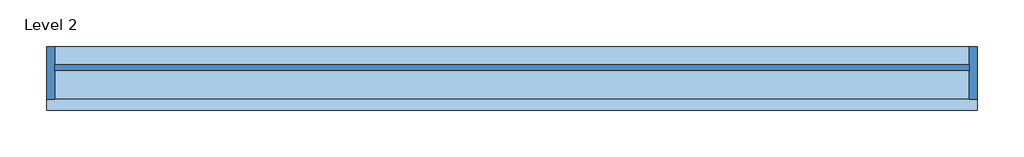
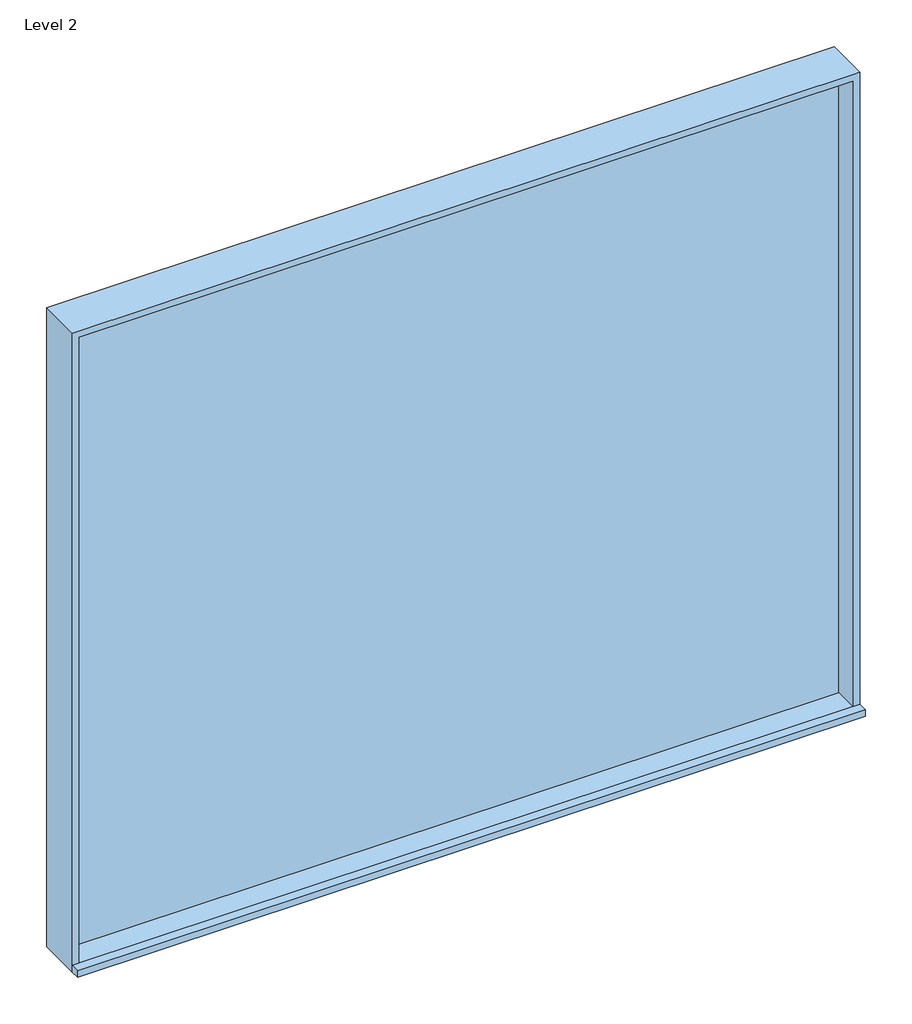
# One storey: 1 window.
"""IFC4 building model written with IfcOpenShell, lengths in millimetres."""

from ifc_helpers import new_model, si_unit, origin, place, context, project, spatial, transform, mapped, element, save
from components import window_88b07bfa

model = new_model("IFC4")

# Units and contexts
model_context = context("Model", 3, world=origin())
ifc_project = project(units=[si_unit("LENGTHUNIT", "METRE", prefix="MILLI")], contexts=[model_context])

# Site, building, storey
site = spatial("IfcSite", under=ifc_project)
building = spatial("IfcBuilding", under=site)
storey = spatial("IfcBuildingStorey", under=building, Name="Level 2", Elevation=3048.0)

# Window
placement = place(None, origin())
window_shape = window_88b07bfa(model_context)
element("IfcWindow", 1, ObjectType="Instance - Fixed : 24\" x 48\"", at=placement, inside=storey, context=model_context, shape_type="MappedRepresentation", body=[
    mapped(window_shape, transform((-10747.8874719, -885.9632813, 3291.4483945), x_axis=(-1.0, 0.0, 0.0), y_axis=(0.0, -1.0, 0.0), z_axis=(0.0, 0.0, 1.0))),
])

save(model, "model.ifc")

# Revit data of these elements
# Type "Instance - Fixed : 24\" x 48\""
#   Type Mark = "10"
#   Construction Type Id = "GSP4R"
#   Assembly Code = "B2020100"
#   Analytic Construction = "1/8 in Pilkington single glazing"
#   Visual Light Transmittance = 0.9
#   Thermal Resistance (R) = 0.8466 (h·ft²·°F)/BTU
#   Solar Heat Gain Coefficient = 0.86
#   Heat Transfer Coefficient (U) = 1.1812 BTU/(h·ft²·°F)
#   Height [instance default] = 4' - 0"
#   Default Sill Height = 3' - 0"
#   Width [instance default] = 2' - 0"
#   Window Inset = 0' - 2"
#   Define Thermal Properties by = 1
#   Glass Pane Material = Glass
#   Sash Material = Iron, Ductile
#   Wall Closure = (empty or 0)
# Element 1 (IfcWindow, "Instance - Fixed : 24\" x 48\"")
#   Mark = "2"
#   Width = 7' - 0"
#   Height = 6' - 0"
#   Phase Created = New Construction
#   Materials on its faces: "Iron, Ductile", "Glass"
# Materials
#   "Glass": class "Glass", colour RGB 0 128 192, transparency 0.75, Description = "Soda Lime Glass", Cost = 0
#   "Iron, Ductile": class "Metal", colour RGB 0 0 0, transparency 0, Description = "Ductile cast iron", Cost = 0
